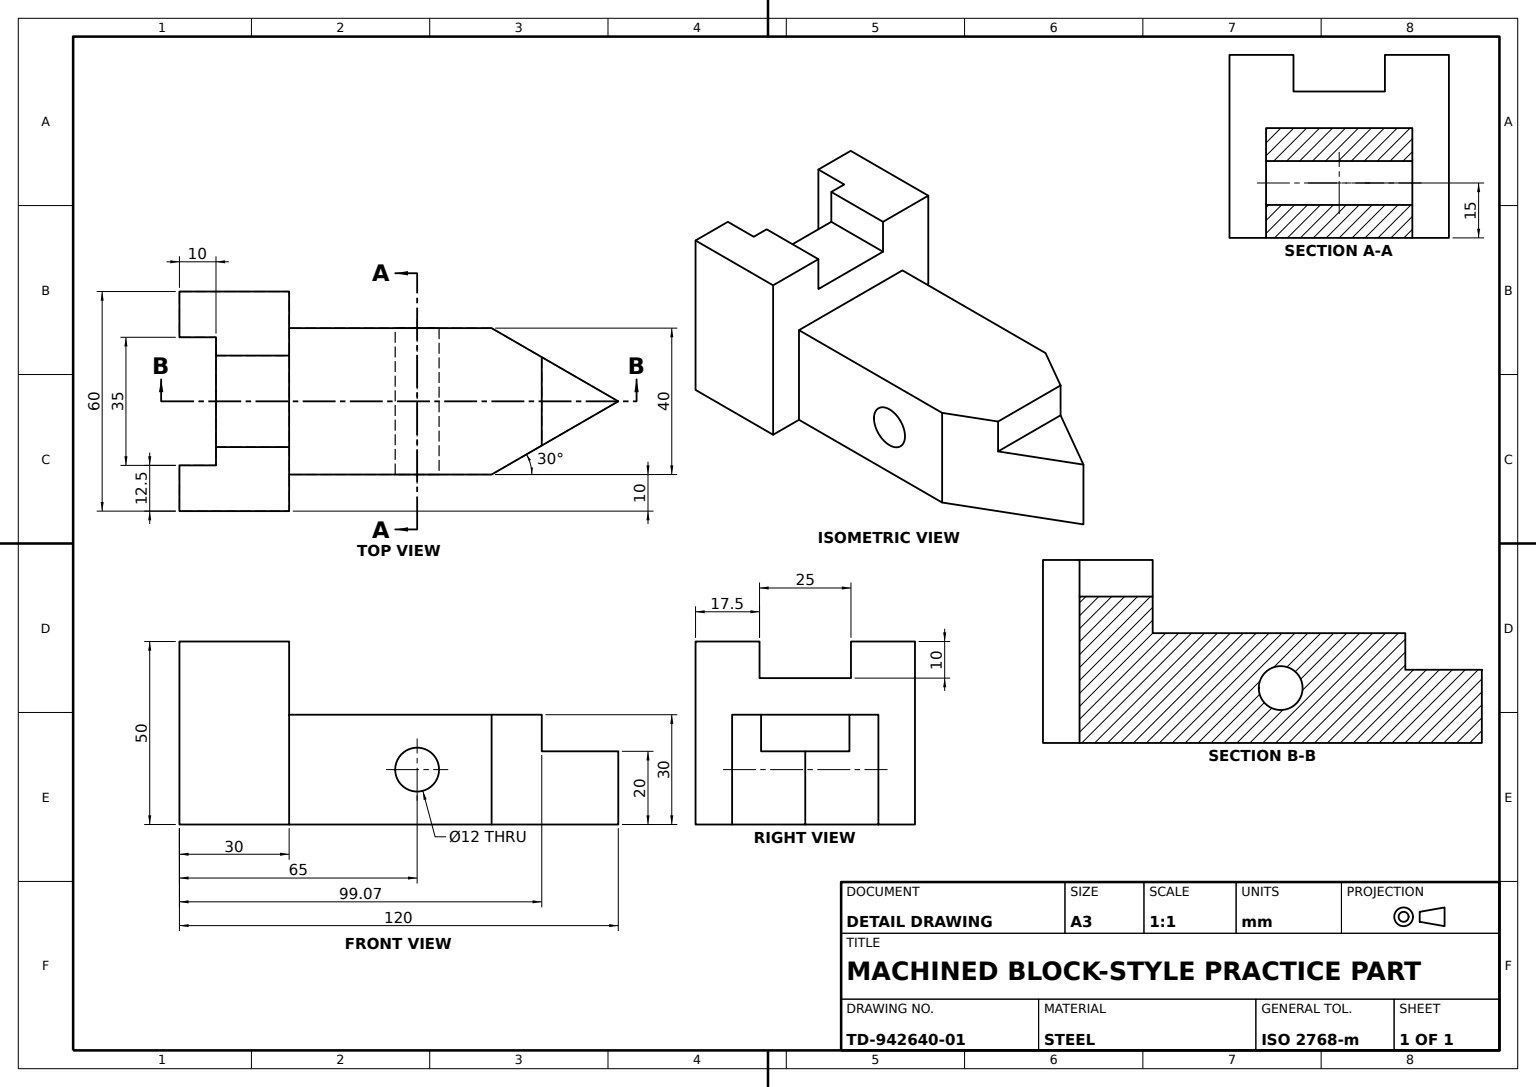
SolidWorks part; units mm, degrees
material "Plain Carbon Steel"
ref_plane "Front Plane" through (0, 0, 0) normal (0, 0, 1) x (1, 0, 0)
ref_plane "Top Plane" through (0, 0, 0) normal (0, 1, 0) x (1, 0, 0)
ref_plane "Right Plane" through (0, 0, 0) normal (1, 0, 0) x (0, 0, -1)
sketch "Base Block Sketch" plane through (0, 0, 0) normal (0, 0, 1) x (1, 0, 0)
  line L1 (0, 0) -> (30, 0)
  line L2 (0, 0) -> (0, 50)
  line L3 (0, 50) -> (30, 50)
  line L4 (30, 0) -> (30, 50)
  dimension "D1" = 30
  dimension "D2" = 50
extrude "Base Block" add sketch "Base Block Sketch" along normal mid plane 60
sketch "Through Slot Sketch" plane through (0, 50, 0) normal (0, 1, 0) x (1, 0, 0)
  line L0 (0, -30) -> (0, 30) construction
  line L1 (0, 17.5) -> (10, 17.5)
  line L2 (0, 17.5) -> (0, -17.5)
  line L3 (0, -17.5) -> (10, -17.5)
  line L4 (10, 17.5) -> (10, -17.5)
  dimension "D1" = 10
  dimension "D2" = 17.5
  dimension "D3" = 35
extrude "Through Slot" cut sketch "Through Slot Sketch" against normal blind 60
sketch "Step Notch Sketch" plane through (30, 0, 0) normal (1, 0, 0) x (0, 0, -1)
  line L0 (0, 0) -> (0, 60.0695) construction
  line L1 (-30, 50) -> (30, 50) construction
  line L2 (-12.5, 50) -> (12.5, 50)
  line L3 (-12.5, 50) -> (-12.5, 40)
  line L4 (-12.5, 40) -> (12.5, 40)
  line L5 (12.5, 50) -> (12.5, 40)
  dimension "D1" = 25
  dimension "D2" = 12.5
  dimension "D3" = 10
extrude "Step Notch" cut sketch "Step Notch Sketch" against normal blind 60
sketch "Nose Boss Sketch" plane through (30, 0, 0) normal (1, 0, 0) x (0, 0, -1)
  line L0 (0, 0) -> (0, 50.7273) construction
  line L1 (-20, 30) -> (20, 30)
  line L2 (20, 30) -> (20, 0)
  line L3 (-30, 0) -> (30, 0) construction
  line L4 (20, 0) -> (-20, 0)
  line L5 (-20, 0) -> (-20, 30)
  dimension "D1" = 20
  dimension "D2" = 40
  dimension "D3" = 30
extrude "Nose Boss" add sketch "Nose Boss Sketch" along normal blind 90
sketch "Corner Cut Sketch" plane through (0, 0, 20) normal (0, 0, 1) x (1, 0, 0)
  line L0 (30, 0) -> (65, 0) construction
  line L1 (120, 0) -> (30, 0) construction
  line L2 (65, 0) -> (65, 15) construction
  circle A0 centre (65, 15) radius 6
  dimension "D3" = 12
  dimension "D1" = 35
  dimension "D2" = 15
extrude "Corner Cut" cut sketch "Corner Cut Sketch" against normal blind 60
sketch "Nose Taper 30deg Sketch" plane through (0, 30, 0) normal (0, 1, 0) x (1, 0, 0)
  line L0 (0, 0) -> (130.3327, 0) construction
  line L1 (75, 36.0262) -> (75, -33.0415) construction
  line L2 (120, 20) -> (120, -20) construction
  line L4 (120, -20) -> (30, -20) construction
  line L6 (120, -20) -> (75, -20)
  line L7 (120, 20) -> (30, 20) construction
  line L8 (75, -20) -> (75, -25.1582)
  line L10 (120, 20) -> (120, -20)
  line L11 (120, 20) -> (99.0745, 20)
  line L12 (99.0745, 20) -> (99.0745, -20)
  line L13 (99.0745, -20) -> (120, -20)
  line L14 (120, 0) -> (99.0745, 12.0813)
  line L15 (120, 0) -> (99.0745, -12.0813)
  line L16 (30, 20) -> (30, -20) construction
  dimension "D1" = 45
  dimension "D2" = 30
  dimension "D3" = 20
  dimension "D4" = 69.0745
  dimension "D5" = 5.1582
extrude "Nose Taper 30deg Cut" cut sketch "Nose Taper 30deg Sketch" against normal blind 60 contours L14 L10 L12 | L11 L15 L12 L6
sketch "Side Pocket Sketch" plane through (0, 30, 0) normal (0, 1, 0) x (1, 0, 0)
  line L0 (99.0745, 12.0813) -> (99.0745, -12.0813)
  line L5 (99.0745, 12.0813) -> (121.0874, 12.0813)
  line L6 (121.0874, 12.0813) -> (121.0874, -12.0813)
  line L7 (121.0874, -12.0813) -> (99.0745, -12.0813)
  dimension "D1" = 22.0128
  dimension "D2" = 24.1626
  dimension "D3" = 99.0745
  dimension "D4" = 12.0813
extrude "Side Pocket 10mm" cut sketch "Side Pocket Sketch" against normal blind 10
sketch "Nose Profile Sketch" plane through (0, 30, 0) normal (0, 1, 0) x (1, 0, 0)
  line L0 (120, 0) -> (99.0745, -12.0813) construction
  line L1 (99.0745, -12.0813) -> (85.359, -20)
  line L2 (85.359, 20) -> (99.0745, 20)
  line L3 (0, 0) -> (127.3932, 0) construction
  line L4 (30, -20) -> (99.0745, -20)
  line L5 (99.0745, -20) -> (99.0745, 20)
  line L6 (99.0745, 20) -> (30, 20)
  line L7 (30, 20) -> (30, -20)
  line L8 (85.359, -20) -> (99.0745, -20)
  line L9 (99.0745, -20) -> (99.0745, 20)
  line L10 (99.0745, 20) -> (85.359, 20)
  line L12 (99.0745, 12.0813) -> (85.359, 20)
  line L13 (85.359, 20) -> (85.359, -20)
  line L14 (85.359, -20) -> (99.0745, -20)
  line M9 (30, -20) -> (99.0745, -20)
  line M10 (99.0745, -20) -> (99.0745, 20)
  line M11 (99.0745, 20) -> (30, 20)
  dimension "D1" = 0
extrude "Nose Profile Cut" cut sketch "Nose Profile Sketch" against normal blind 30 contours L12 L9 M11 | L1 M10 M9
